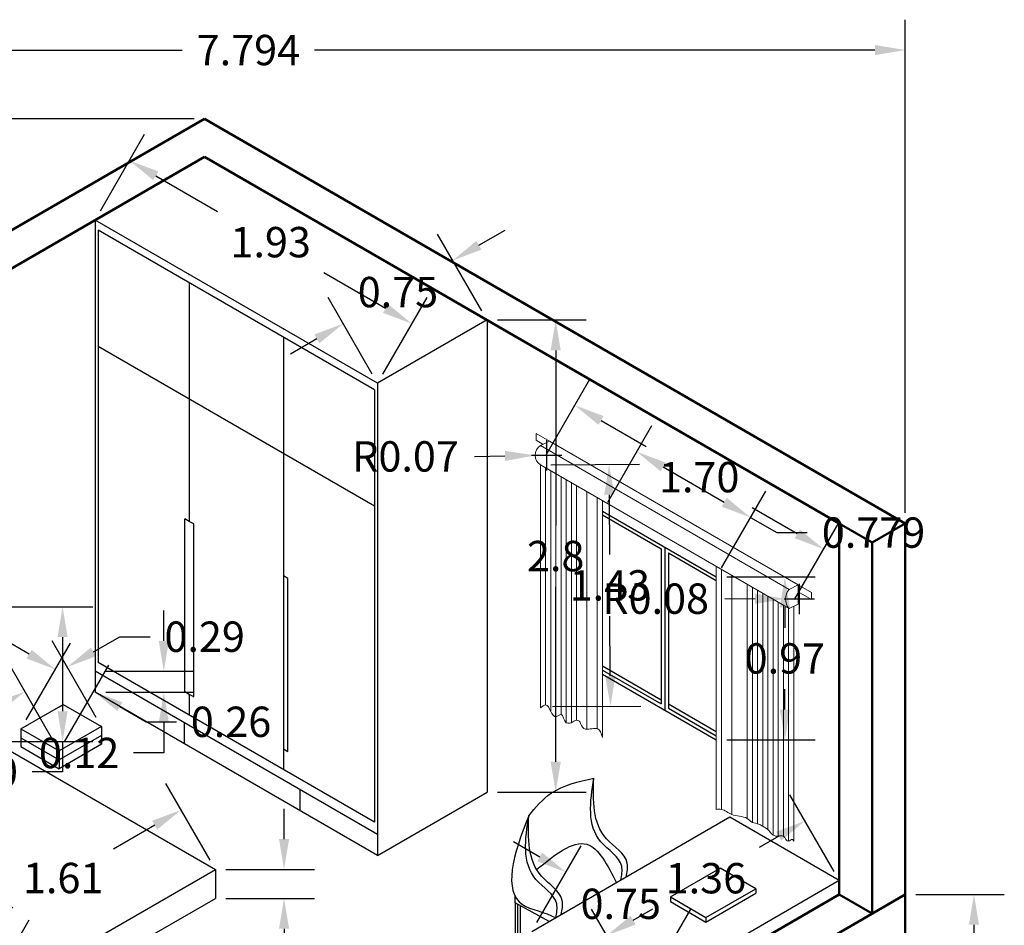
# Model space of a CAD drawing. Units: metres. Extents: x 4633 to 4644.7, y 5356.8 to 5365.2.
# Tile 3 of 3: x 4638.8 to 4644.7, y 5359.9 to 5365.2. Entities that reach past the tile are written whole.
import ezdxf

# ---------------------------------------------------------------- set-up
doc = ezdxf.new("R2010")
doc.units = ezdxf.units.M
for name, color, linetype, lineweight in [('A-ANNO-DIMS', 2, 'Continuous', 18), ('A-FURN', 8, 'Continuous', 25), ('A-FURN-CURT', 8, 'Continuous', 18), ('A-GLAZ', 4, 'Continuous', 25), ('A-WALL', 7, 'Continuous', 50)]:
    doc.layers.add(name, color=color, linetype=linetype, lineweight=lineweight)
doc.styles.get("Standard").update_dxf_attribs({"font": 'arial.ttf'})
doc.dimstyles.get("Standard").update_dxf_attribs({"dimtxt": 0.18, "dimasz": 0.18, "dimexe": 0.18, "dimexo": 0.0625, "dimgap": 0.09, "dimtad": 0, "dimtih": 1, "dimtoh": 1, "dimdec": 4, "dimzin": 0, "dimdsep": 46, "dimtxsty": 'Standard', "dimcen": 0.09, "dimadec": 0, "dimazin": 0, "dimtfac": 1, "dimtdec": 4, "dimtofl": 0, "dimtmove": 0, "dimatfit": 3, "dimfxl": 1, "dimtolj": 1, "dimtzin": 0, "dimarcsym": 0})

# ---------------------------------------------------------------- blocks, each defined once
blk = doc.blocks.new('*D2')
at = {"layer": 'A-ANNO-DIMS', "color": 0, "lineweight": -2, "transparency": 16777216}
for p, q in [((4636.2802, 5362.6038), (4636.2802, 5365.2288)), ((4644.0744, 5362.3038), (4644.0744, 5365.2288)), ((4636.4602, 5365.0488), (4639.7847, 5365.0488)), ((4643.8944, 5365.0488), (4640.5699, 5365.0488))]:
    blk.add_line(p, q, dxfattribs=at)
at = {"layer": 'A-ANNO-DIMS', "color": 0, "transparency": 16777216}
for points in [[(4636.4602, 5365.0788), (4636.4602, 5365.0188), (4636.2802, 5365.0488)], [(4643.8944, 5365.0788), (4643.8944, 5365.0188), (4644.0744, 5365.0488)]]:
    blk.add_solid(points, dxfattribs=at)
at = {"layer": 'Defpoints', "color": 0, "transparency": 16777216}
for p in [(4644.0744, 5365.0488), (4636.2802, 5362.5413), (4644.0744, 5362.2413)]:
    blk.add_point(p, dxfattribs=at)
at = {"layer": 'A-ANNO-DIMS', "color": 0, "transparency": 16777216, "insert": (4640.1773, 5365.0488), "char_height": 0.18, "attachment_point": 5}
blk.add_mtext('\\A1;7.794', dxfattribs=at)
blk = doc.blocks.new('*D3')
at = {"layer": 'A-ANNO-DIMS', "color": 0, "lineweight": -2, "transparency": 16777216}
for p, q in [((4639.855, 5364.6413), (4635.6927, 5364.6413)), ((4635.8727, 5364.4613), (4635.8727, 5360.9232)), ((4635.8727, 5357.0213), (4635.8727, 5360.5594)), ((4639.855, 5356.8413), (4635.6927, 5356.8413))]:
    blk.add_line(p, q, dxfattribs=at)
at = {"layer": 'A-ANNO-DIMS', "color": 0, "transparency": 16777216}
for points in [[(4635.8427, 5364.4613), (4635.9027, 5364.4613), (4635.8727, 5364.6413)], [(4635.8427, 5357.0213), (4635.9027, 5357.0213), (4635.8727, 5356.8413)]]:
    blk.add_solid(points, dxfattribs=at)
at = {"layer": 'Defpoints', "color": 0, "transparency": 16777216}
for p in [(4639.9175, 5364.6413), (4635.8727, 5356.8413), (4639.9175, 5356.8413)]:
    blk.add_point(p, dxfattribs=at)
at = {"layer": 'A-ANNO-DIMS', "color": 0, "transparency": 16777216, "insert": (4635.8727, 5360.7413), "char_height": 0.18, "attachment_point": 5}
blk.add_mtext('\\A1;7.8', dxfattribs=at)
blk = doc.blocks.new('*D6')
at = {"layer": 'A-ANNO-DIMS', "color": 0, "lineweight": -2, "transparency": 16777216}
for p, q in [((4644.1369, 5360.0413), (4644.6619, 5360.0413)), ((4644.4819, 5359.8613), (4644.4819, 5359.4213)), ((4644.1369, 5359.2413), (4644.6619, 5359.2413)), ((4644.4819, 5359.2413), (4644.4819, 5359.0613)), ((4644.4819, 5359.0613), (4644.3019, 5359.0613))]:
    blk.add_line(p, q, dxfattribs=at)
at = {"layer": 'A-ANNO-DIMS', "color": 0, "transparency": 16777216}
for points in [[(4644.4519, 5359.8613), (4644.5119, 5359.8613), (4644.4819, 5360.0413)], [(4644.4519, 5359.4213), (4644.5119, 5359.4213), (4644.4819, 5359.2413)]]:
    blk.add_solid(points, dxfattribs=at)
at = {"layer": 'Defpoints', "color": 0, "transparency": 16777216}
for p in [(4644.0744, 5360.0413), (4644.0744, 5359.2413), (4644.4819, 5359.2413)]:
    blk.add_point(p, dxfattribs=at)
at = {"layer": 'A-ANNO-DIMS', "color": 0, "transparency": 16777216, "insert": (4644.0479, 5359.0613), "char_height": 0.18, "attachment_point": 5}
blk.add_mtext('\\A1;0.8', dxfattribs=at)
blk = doc.blocks.new('*D9')
at = {"layer": 'A-ANNO-DIMS', "color": 0, "lineweight": -2, "transparency": 16777216}
for p, q in [((4642.309, 5362.3679), (4642.5715, 5362.8225)), ((4642.6374, 5362.5767), (4643.0003, 5362.3671)), ((4642.9837, 5361.9783), (4643.2462, 5362.433)), ((4643.1562, 5362.2771), (4643.3121, 5362.1871)), ((4643.3121, 5362.1871), (4643.4921, 5362.1871))]:
    blk.add_line(p, q, dxfattribs=at)
at = {"layer": 'A-ANNO-DIMS', "color": 0, "transparency": 16777216}
for points in [[(4642.6524, 5362.6026), (4642.6224, 5362.5507), (4642.4815, 5362.6667)], [(4643.0153, 5362.3931), (4642.9853, 5362.3411), (4643.1562, 5362.2771)]]:
    blk.add_solid(points, dxfattribs=at)
at = {"layer": 'Defpoints', "color": 0, "transparency": 16777216}
for p in [(4642.2778, 5362.3137), (4643.1562, 5362.2771), (4642.9525, 5361.9242)]:
    blk.add_point(p, dxfattribs=at)
at = {"layer": 'A-ANNO-DIMS', "color": 0, "transparency": 16777216, "insert": (4643.886, 5362.1871), "char_height": 0.18, "attachment_point": 5}
blk.add_mtext('\\A1;0.779', dxfattribs=at)
blk = doc.blocks.new('*D10')
at = {"layer": 'A-ANNO-DIMS', "color": 0, "lineweight": -2, "transparency": 16777216}
for p, q in [((4643.015, 5361.9242), (4643.54, 5361.9242)), ((4643.36, 5361.7442), (4643.36, 5361.6227)), ((4643.36, 5361.1374), (4643.36, 5361.2589)), ((4643.015, 5360.9574), (4643.54, 5360.9574))]:
    blk.add_line(p, q, dxfattribs=at)
at = {"layer": 'A-ANNO-DIMS', "color": 0, "transparency": 16777216}
for points in [[(4643.33, 5361.7442), (4643.39, 5361.7442), (4643.36, 5361.9242)], [(4643.33, 5361.1374), (4643.39, 5361.1374), (4643.36, 5360.9574)]]:
    blk.add_solid(points, dxfattribs=at)
at = {"layer": 'Defpoints', "color": 0, "transparency": 16777216}
for p in [(4642.9525, 5361.9242), (4642.9525, 5360.9574), (4643.36, 5360.9574)]:
    blk.add_point(p, dxfattribs=at)
at = {"layer": 'A-ANNO-DIMS', "color": 0, "transparency": 16777216, "insert": (4643.36, 5361.4408), "char_height": 0.18, "attachment_point": 5}
blk.add_mtext('\\A1;0.97', dxfattribs=at)
blk = doc.blocks.new('*D11')
at = {"layer": 'A-ANNO-DIMS', "color": 0, "lineweight": -2, "transparency": 16777216}
for p, q in [((4641.9722, 5362.5896), (4642.4972, 5362.5926)), ((4642.3183, 5362.4116), (4642.3203, 5362.0563)), ((4642.3243, 5361.337), (4642.3223, 5361.6923)), ((4641.9804, 5361.1551), (4642.5054, 5361.158))]:
    blk.add_line(p, q, dxfattribs=at)
at = {"layer": 'A-ANNO-DIMS', "color": 0, "transparency": 16777216}
for points in [[(4642.3483, 5362.4117), (4642.2883, 5362.4114), (4642.3172, 5362.5916)], [(4642.3543, 5361.3372), (4642.2943, 5361.3368), (4642.3254, 5361.157)]]:
    blk.add_solid(points, dxfattribs=at)
at = {"layer": 'Defpoints', "color": 0, "transparency": 16777216}
for p in [(4641.9097, 5362.5893), (4642.3254, 5361.157), (4641.9179, 5361.1547)]:
    blk.add_point(p, dxfattribs=at)
at = {"layer": 'A-ANNO-DIMS', "color": 0, "transparency": 16777216, "insert": (4642.3213, 5361.8743), "char_height": 0.18, "attachment_point": 5}
blk.add_mtext('\\A1;1.43', dxfattribs=at)
blk = doc.blocks.new('*D12')
at = {"layer": 'A-ANNO-DIMS', "color": 0, "lineweight": -2, "transparency": 16777216}
for p, q in [((4641.941, 5362.6434), (4642.2035, 5363.098)), ((4642.2694, 5362.8522), (4642.5366, 5362.6979)), ((4643.4339, 5362.1798), (4643.1666, 5362.3341)), ((4643.4173, 5361.791), (4643.6798, 5362.2457))]:
    blk.add_line(p, q, dxfattribs=at)
at = {"layer": 'A-ANNO-DIMS', "color": 0, "transparency": 16777216}
for points in [[(4642.2844, 5362.8781), (4642.2544, 5362.8262), (4642.1135, 5362.9422)], [(4643.4489, 5362.2058), (4643.4189, 5362.1538), (4643.5898, 5362.0898)]]:
    blk.add_solid(points, dxfattribs=at)
at = {"layer": 'Defpoints', "color": 0, "transparency": 16777216}
for p in [(4641.9097, 5362.5893), (4643.5898, 5362.0898), (4643.386, 5361.7369)]:
    blk.add_point(p, dxfattribs=at)
at = {"layer": 'A-ANNO-DIMS', "color": 0, "transparency": 16777216, "insert": (4642.8516, 5362.516), "char_height": 0.18, "attachment_point": 5}
blk.add_mtext('\\A1;1.70', dxfattribs=at)
blk = doc.blocks.new('*D13')
at = {"layer": 'A-ANNO-DIMS', "color": 0, "lineweight": -2, "transparency": 16777216}
for p, q in [((4639.2992, 5364.0944), (4639.5617, 5364.5491)), ((4639.6276, 5364.3032), (4639.9942, 5364.0915)), ((4640.9911, 5363.516), (4640.6245, 5363.7276)), ((4640.9745, 5363.1272), (4641.237, 5363.5818))]:
    blk.add_line(p, q, dxfattribs=at)
at = {"layer": 'A-ANNO-DIMS', "color": 0, "transparency": 16777216}
for points in [[(4639.6426, 5364.3292), (4639.6126, 5364.2772), (4639.4717, 5364.3932)], [(4641.0061, 5363.5419), (4640.9761, 5363.49), (4641.147, 5363.426)]]:
    blk.add_solid(points, dxfattribs=at)
at = {"layer": 'Defpoints', "color": 0, "transparency": 16777216}
for p in [(4639.268, 5364.0403), (4641.147, 5363.426), (4640.9433, 5363.073)]:
    blk.add_point(p, dxfattribs=at)
at = {"layer": 'A-ANNO-DIMS', "color": 0, "transparency": 16777216, "insert": (4640.3094, 5363.9096), "char_height": 0.18, "attachment_point": 5}
blk.add_mtext('\\A1;1.93', dxfattribs=at)
blk = doc.blocks.new('*D14')
at = {"layer": 'A-ANNO-DIMS', "color": 0, "lineweight": -2, "transparency": 16777216}
for p, q in [((4641.5449, 5363.891), (4641.7008, 5363.981)), ((4641.5615, 5363.5022), (4641.299, 5363.9568)), ((4640.912, 5363.1272), (4640.6495, 5363.5818)), ((4640.5836, 5363.336), (4640.4277, 5363.246))]:
    blk.add_line(p, q, dxfattribs=at)
at = {"layer": 'A-ANNO-DIMS', "color": 0, "transparency": 16777216}
for points in [[(4641.5299, 5363.9169), (4641.5599, 5363.865), (4641.389, 5363.801)], [(4640.5686, 5363.3619), (4640.5986, 5363.31), (4640.7395, 5363.426)]]:
    blk.add_solid(points, dxfattribs=at)
at = {"layer": 'Defpoints', "color": 0, "transparency": 16777216}
for p in [(4641.389, 5363.801), (4641.5928, 5363.448), (4640.9433, 5363.073)]:
    blk.add_point(p, dxfattribs=at)
at = {"layer": 'A-ANNO-DIMS', "color": 0, "transparency": 16777216, "insert": (4641.0643, 5363.6135), "char_height": 0.18, "attachment_point": 5}
blk.add_mtext('\\A1;0.75', dxfattribs=at)
blk = doc.blocks.new('*D15')
at = {"layer": 'A-ANNO-DIMS', "color": 0, "lineweight": -2, "transparency": 16777216}
for p, q in [((4641.6553, 5363.448), (4642.1803, 5363.448)), ((4642.0003, 5363.268), (4642.0003, 5362.23)), ((4642.0003, 5360.828), (4642.0003, 5361.8661)), ((4641.6553, 5360.648), (4642.1803, 5360.648))]:
    blk.add_line(p, q, dxfattribs=at)
at = {"layer": 'A-ANNO-DIMS', "color": 0, "transparency": 16777216}
for points in [[(4641.9703, 5363.268), (4642.0303, 5363.268), (4642.0003, 5363.448)], [(4641.9703, 5360.828), (4642.0303, 5360.828), (4642.0003, 5360.648)]]:
    blk.add_solid(points, dxfattribs=at)
at = {"layer": 'Defpoints', "color": 0, "transparency": 16777216}
for p in [(4641.5928, 5363.448), (4641.5928, 5360.648), (4642.0003, 5360.648)]:
    blk.add_point(p, dxfattribs=at)
at = {"layer": 'A-ANNO-DIMS', "color": 0, "transparency": 16777216, "insert": (4642.0003, 5362.048), "char_height": 0.18, "attachment_point": 5}
blk.add_mtext('\\A1;2.8', dxfattribs=at)
blk = doc.blocks.new('*D16')
at = {"layer": 'A-ANNO-DIMS', "color": 0, "lineweight": -2, "transparency": 16777216}
for p, q in [((4639.6755, 5361.545), (4639.6755, 5361.725)), ((4639.3305, 5361.365), (4639.8555, 5361.365)), ((4639.3305, 5361.2403), (4639.8555, 5361.2403)), ((4639.6755, 5361.0603), (4639.6755, 5360.8803)), ((4639.6755, 5360.8803), (4639.4955, 5360.8803))]:
    blk.add_line(p, q, dxfattribs=at)
at = {"layer": 'A-ANNO-DIMS', "color": 0, "transparency": 16777216}
for points in [[(4639.6455, 5361.545), (4639.7055, 5361.545), (4639.6755, 5361.365)], [(4639.6455, 5361.0603), (4639.7055, 5361.0603), (4639.6755, 5361.2403)]]:
    blk.add_solid(points, dxfattribs=at)
at = {"layer": 'Defpoints', "color": 0, "transparency": 16777216}
for p in [(4639.268, 5361.365), (4639.268, 5361.2403), (4639.6755, 5361.2403)]:
    blk.add_point(p, dxfattribs=at)
at = {"layer": 'A-ANNO-DIMS', "color": 0, "transparency": 16777216, "insert": (4639.1726, 5360.8803), "char_height": 0.18, "attachment_point": 5}
blk.add_mtext('\\A1;0.12', dxfattribs=at)
blk = doc.blocks.new('*D17')
at = {"layer": 'A-ANNO-DIMS', "color": 0, "lineweight": -2, "transparency": 16777216}
for p, q in [((4637.213, 5360.2454), (4637.4755, 5360.7001)), ((4637.5414, 5360.4542), (4637.771, 5360.3216)), ((4638.6308, 5359.8252), (4638.4012, 5359.9578)), ((4638.6142, 5359.4364), (4638.8767, 5359.8911))]:
    blk.add_line(p, q, dxfattribs=at)
at = {"layer": 'A-ANNO-DIMS', "color": 0, "transparency": 16777216}
for points in [[(4637.5564, 5360.4802), (4637.5264, 5360.4282), (4637.3855, 5360.5442)], [(4638.6458, 5359.8512), (4638.6158, 5359.7992), (4638.7867, 5359.7352)]]:
    blk.add_solid(points, dxfattribs=at)
at = {"layer": 'Defpoints', "color": 0, "transparency": 16777216}
for p in [(4637.1817, 5360.1913), (4638.7867, 5359.7352), (4638.583, 5359.3823)]:
    blk.add_point(p, dxfattribs=at)
at = {"layer": 'A-ANNO-DIMS', "color": 0, "transparency": 16777216, "insert": (4638.0861, 5360.1397), "char_height": 0.18, "attachment_point": 5}
blk.add_mtext('\\A1;1.618', dxfattribs=at)
blk = doc.blocks.new('*D18')
at = {"layer": 'A-ANNO-DIMS', "color": 0, "lineweight": -2, "transparency": 16777216}
for p, q in [((4639.9499, 5360.2437), (4639.6874, 5360.6983)), ((4639.6215, 5360.4524), (4639.3762, 5360.3108)), ((4638.5351, 5359.8252), (4638.7804, 5359.9668)), ((4638.5517, 5359.4364), (4638.2892, 5359.8911))]:
    blk.add_line(p, q, dxfattribs=at)
at = {"layer": 'A-ANNO-DIMS', "color": 0, "transparency": 16777216}
for points in [[(4639.6065, 5360.4784), (4639.6365, 5360.4265), (4639.7774, 5360.5424)], [(4638.5201, 5359.8512), (4638.5501, 5359.7992), (4638.3792, 5359.7352)]]:
    blk.add_solid(points, dxfattribs=at)
at = {"layer": 'Defpoints', "color": 0, "transparency": 16777216}
for p in [(4639.7774, 5360.5424), (4639.9812, 5360.1895), (4638.583, 5359.3823)]:
    blk.add_point(p, dxfattribs=at)
at = {"layer": 'A-ANNO-DIMS', "color": 0, "transparency": 16777216, "insert": (4639.0783, 5360.1388), "char_height": 0.18, "attachment_point": 5}
blk.add_mtext('\\A1;1.61', dxfattribs=at)
blk = doc.blocks.new('*D19')
at = {"layer": 'A-ANNO-DIMS', "color": 0, "lineweight": -2, "transparency": 16777216}
for p, q in [((4640.3887, 5360.3695), (4640.3887, 5360.5495)), ((4640.0437, 5360.1895), (4640.5687, 5360.1895)), ((4640.0437, 5360.0182), (4640.5687, 5360.0182)), ((4640.3887, 5359.8382), (4640.3887, 5359.6582)), ((4640.3887, 5359.6582), (4640.2087, 5359.6582))]:
    blk.add_line(p, q, dxfattribs=at)
at = {"layer": 'A-ANNO-DIMS', "color": 0, "transparency": 16777216}
for points in [[(4640.3587, 5360.3695), (4640.4187, 5360.3695), (4640.3887, 5360.1895)], [(4640.3587, 5359.8382), (4640.4187, 5359.8382), (4640.3887, 5360.0182)]]:
    blk.add_solid(points, dxfattribs=at)
at = {"layer": 'Defpoints', "color": 0, "transparency": 16777216}
for p in [(4639.9812, 5360.1895), (4639.9812, 5360.0182), (4640.3887, 5360.0182)]:
    blk.add_point(p, dxfattribs=at)
at = {"layer": 'A-ANNO-DIMS', "color": 0, "transparency": 16777216, "insert": (4639.8849, 5359.6582), "char_height": 0.18, "attachment_point": 5}
blk.add_mtext('\\A1;0.17', dxfattribs=at)
blk = doc.blocks.new('*D20')
at = {"layer": 'A-ANNO-DIMS', "color": 0, "lineweight": -2, "transparency": 16777216}
for p, q in [((4638.7298, 5361.7474), (4639.2548, 5361.7474)), ((4639.0748, 5361.5674), (4639.0748, 5361.1281)), ((4638.7298, 5360.9481), (4639.2548, 5360.9481)), ((4639.0748, 5360.9481), (4639.0748, 5360.7681)), ((4639.0748, 5360.7681), (4638.8948, 5360.7681))]:
    blk.add_line(p, q, dxfattribs=at)
at = {"layer": 'A-ANNO-DIMS', "color": 0, "transparency": 16777216}
for points in [[(4639.0448, 5361.5674), (4639.1048, 5361.5674), (4639.0748, 5361.7474)], [(4639.0448, 5361.1281), (4639.1048, 5361.1281), (4639.0748, 5360.9481)]]:
    blk.add_solid(points, dxfattribs=at)
at = {"layer": 'Defpoints', "color": 0, "transparency": 16777216}
for p in [(4638.6673, 5361.7474), (4638.6673, 5360.9481), (4639.0748, 5360.9481)]:
    blk.add_point(p, dxfattribs=at)
at = {"layer": 'A-ANNO-DIMS', "color": 0, "transparency": 16777216, "insert": (4638.5714, 5360.7681), "char_height": 0.18, "attachment_point": 5}
blk.add_mtext('\\A1;0.80', dxfattribs=at)
blk = doc.blocks.new('*D22')
at = {"layer": 'A-ANNO-DIMS', "color": 0, "lineweight": -2, "transparency": 16777216}
for p, q in [((4638.8758, 5361.4662), (4638.7199, 5361.5562)), ((4638.8591, 5361.0775), (4639.1216, 5361.5321)), ((4639.0863, 5360.9463), (4639.3488, 5361.401)), ((4639.4147, 5361.1551), (4639.5706, 5361.0651)), ((4639.5706, 5361.0651), (4639.7506, 5361.0651))]:
    blk.add_line(p, q, dxfattribs=at)
at = {"layer": 'A-ANNO-DIMS', "color": 0, "transparency": 16777216}
for points in [[(4638.8908, 5361.4922), (4638.8608, 5361.4403), (4639.0316, 5361.3762)], [(4639.4297, 5361.1811), (4639.3997, 5361.1291), (4639.2588, 5361.2451)]]:
    blk.add_solid(points, dxfattribs=at)
at = {"layer": 'Defpoints', "color": 0, "transparency": 16777216}
for p in [(4639.2588, 5361.2451), (4638.8279, 5361.0233), (4639.0551, 5360.8922)]:
    blk.add_point(p, dxfattribs=at)
at = {"layer": 'A-ANNO-DIMS', "color": 0, "transparency": 16777216, "insert": (4640.0743, 5361.0651), "char_height": 0.18, "attachment_point": 5}
blk.add_mtext('\\A1;0.26', dxfattribs=at)
blk = doc.blocks.new('*D23')
at = {"layer": 'A-ANNO-DIMS', "color": 0, "lineweight": -2, "transparency": 16777216}
for p, q in [((4639.258, 5361.4799), (4639.4139, 5361.5699)), ((4639.4139, 5361.5699), (4639.5939, 5361.5699)), ((4639.2746, 5361.0911), (4639.0121, 5361.5457)), ((4639.0238, 5360.9463), (4638.7613, 5361.401)), ((4638.6954, 5361.1551), (4638.5395, 5361.0651))]:
    blk.add_line(p, q, dxfattribs=at)
at = {"layer": 'A-ANNO-DIMS', "color": 0, "transparency": 16777216}
for points in [[(4639.243, 5361.5058), (4639.273, 5361.4539), (4639.1021, 5361.3899)], [(4638.6804, 5361.1811), (4638.7104, 5361.1291), (4638.8513, 5361.2451)]]:
    blk.add_solid(points, dxfattribs=at)
at = {"layer": 'Defpoints', "color": 0, "transparency": 16777216}
for p in [(4639.1021, 5361.3899), (4639.3058, 5361.037), (4639.0551, 5360.8922)]:
    blk.add_point(p, dxfattribs=at)
at = {"layer": 'A-ANNO-DIMS', "color": 0, "transparency": 16777216, "insert": (4639.9178, 5361.5699), "char_height": 0.18, "attachment_point": 5}
blk.add_mtext('\\A1;0.29', dxfattribs=at)
blk = doc.blocks.new('*D25')
at = {"layer": 'A-ANNO-DIMS', "color": 0, "lineweight": -2, "transparency": 16777216}
for p, q in [((4641.9058, 5360.2632), (4641.7499, 5360.3532)), ((4641.8892, 5359.8745), (4642.1517, 5360.3291)), ((4642.5387, 5359.4995), (4642.8012, 5359.9541)), ((4642.8671, 5359.7082), (4643.023, 5359.6182))]:
    blk.add_line(p, q, dxfattribs=at)
at = {"layer": 'A-ANNO-DIMS', "color": 0, "transparency": 16777216}
for points in [[(4641.9208, 5360.2892), (4641.8908, 5360.2373), (4642.0617, 5360.1732)], [(4642.8821, 5359.7342), (4642.8521, 5359.6823), (4642.7112, 5359.7982)]]:
    blk.add_solid(points, dxfattribs=at)
at = {"layer": 'Defpoints', "color": 0, "transparency": 16777216}
for p in [(4641.8579, 5359.8203), (4642.7112, 5359.7982), (4642.5075, 5359.4453)]:
    blk.add_point(p, dxfattribs=at)
at = {"layer": 'A-ANNO-DIMS', "color": 0, "transparency": 16777216, "insert": (4642.3865, 5359.9857), "char_height": 0.18, "attachment_point": 5}
blk.add_mtext('\\A1;0.75', dxfattribs=at)
blk = doc.blocks.new('*D26')
at = {"layer": 'A-ANNO-DIMS', "color": 0, "lineweight": -2, "transparency": 16777216}
for p, q in [((4643.6517, 5360.1781), (4643.3892, 5360.6328)), ((4643.3233, 5360.3869), (4643.2066, 5360.3195)), ((4642.4762, 5359.4995), (4642.2137, 5359.9541)), ((4642.4596, 5359.8882), (4642.5763, 5359.9556))]:
    blk.add_line(p, q, dxfattribs=at)
at = {"layer": 'A-ANNO-DIMS', "color": 0, "transparency": 16777216}
for points in [[(4643.3083, 5360.4129), (4643.3383, 5360.3609), (4643.4792, 5360.4769)], [(4642.4446, 5359.9142), (4642.4746, 5359.8623), (4642.3037, 5359.7982)]]:
    blk.add_solid(points, dxfattribs=at)
at = {"layer": 'Defpoints', "color": 0, "transparency": 16777216}
for p in [(4643.4792, 5360.4769), (4643.683, 5360.124), (4642.5075, 5359.4453)]:
    blk.add_point(p, dxfattribs=at)
at = {"layer": 'A-ANNO-DIMS', "color": 0, "transparency": 16777216, "insert": (4642.8915, 5360.1376), "char_height": 0.18, "attachment_point": 5}
blk.add_mtext('\\A1;1.36', dxfattribs=at)
blk = doc.blocks.new('*D30')
at = {"layer": 'A-ANNO-DIMS', "color": 0, "lineweight": -2, "transparency": 16777216}
for p, q in [((4633.8236, 5361.0144), (4634.0036, 5361.0144)), ((4634.0036, 5361.0144), (4636.779, 5359.9989)), ((4641.8554, 5358.0514), (4641.8554, 5358.2314)), ((4641.7654, 5358.1414), (4641.9454, 5358.1414))]:
    blk.add_line(p, q, dxfattribs=at)
at = {"layer": 'A-ANNO-DIMS', "color": 0, "transparency": 16777216}
blk.add_solid([(4636.7893, 5360.027), (4636.7686, 5359.9707), (4636.948, 5359.937)], dxfattribs=at)
at = {"layer": 'Defpoints', "color": 0, "transparency": 16777216}
for p in [(4636.948, 5359.937), (4641.8554, 5358.1414)]:
    blk.add_point(p, dxfattribs=at)
at = {"layer": 'A-ANNO-DIMS', "color": 0, "transparency": 16777216, "insert": (4633.3438, 5361.0144), "char_height": 0.18, "attachment_point": 5}
blk.add_mtext('\\A1;R5.226', dxfattribs=at)
blk = doc.blocks.new('*D32')
at = {"layer": 'A-ANNO-DIMS', "color": 0, "lineweight": -2, "transparency": 16777216}
for p, q in [((4643.4464, 5361.7037), (4643.4464, 5361.8837)), ((4643.0035, 5361.7954), (4643.1835, 5361.7947)), ((4643.3564, 5361.7937), (4643.5364, 5361.7937))]:
    blk.add_line(p, q, dxfattribs=at)
at = {"layer": 'A-ANNO-DIMS', "color": 0, "transparency": 16777216}
blk.add_solid([(4643.1837, 5361.8247), (4643.1834, 5361.7647), (4643.3635, 5361.794)], dxfattribs=at)
at = {"layer": 'Defpoints', "color": 0, "transparency": 16777216}
for p in [(4643.3635, 5361.794), (4643.4464, 5361.7937)]:
    blk.add_point(p, dxfattribs=at)
at = {"layer": 'A-ANNO-DIMS', "color": 0, "transparency": 16777216, "insert": (4642.5935, 5361.7954), "char_height": 0.18, "attachment_point": 5}
blk.add_mtext('\\A1;R0.08', dxfattribs=at)
blk = doc.blocks.new('*D33')
at = {"layer": 'A-ANNO-DIMS', "color": 0, "lineweight": -2, "transparency": 16777216}
for p, q in [((4641.947, 5362.556), (4641.947, 5362.736)), ((4641.5191, 5362.6391), (4641.6991, 5362.642)), ((4641.857, 5362.646), (4642.037, 5362.646))]:
    blk.add_line(p, q, dxfattribs=at)
at = {"layer": 'A-ANNO-DIMS', "color": 0, "transparency": 16777216}
blk.add_solid([(4641.6986, 5362.672), (4641.6996, 5362.612), (4641.8791, 5362.6449)], dxfattribs=at)
at = {"layer": 'Defpoints', "color": 0, "transparency": 16777216}
for p in [(4641.8791, 5362.6449), (4641.947, 5362.646)]:
    blk.add_point(p, dxfattribs=at)
at = {"layer": 'A-ANNO-DIMS', "color": 0, "transparency": 16777216, "insert": (4641.1092, 5362.6391), "char_height": 0.18, "attachment_point": 5}
blk.add_mtext('\\A1;R0.07', dxfattribs=at)

msp = doc.modelspace()

# ---------------------------------------------------------------- linework, layer by layer
at = {"layer": 'A-FURN'}
for p, q in [((4640.9433, 5363.073), (4639.268, 5364.0403)), ((4639.268, 5364.0403), (4639.268, 5361.2403)), ((4639.2853, 5363.9803), (4639.2853, 5361.4165)), ((4640.9259, 5363.033), (4639.2853, 5363.9803)), ((4639.8264, 5363.6679), (4639.8264, 5362.2537)), ((4641.5928, 5363.448), (4640.9433, 5363.073)), ((4641.5928, 5363.448), (4641.5928, 5360.648)), ((4640.3848, 5363.3455), (4640.3848, 5360.7817)), ((4640.9259, 5362.3435), (4639.2853, 5363.2907)), ((4640.9259, 5363.033), (4640.9259, 5360.4693)), ((4640.9433, 5363.073), (4640.9433, 5360.273)), ((4639.7998, 5361.244), (4639.7998, 5362.2691)), ((4639.8264, 5362.2537), (4639.7998, 5362.2691)), ((4639.853, 5362.2383), (4639.8264, 5362.2537)), ((4639.853, 5361.2133), (4639.853, 5362.2383)), ((4640.4115, 5361.9145), (4640.3848, 5361.9299)), ((4640.4115, 5360.8895), (4640.4115, 5361.9145)), ((4640.9259, 5360.4693), (4639.2853, 5361.4165)), ((4640.9433, 5360.3977), (4639.268, 5361.365)), ((4640.9433, 5360.273), (4639.268, 5361.2403)), ((4639.7998, 5361.244), (4639.8264, 5361.2286)), ((4639.8264, 5361.2286), (4639.853, 5361.2133)), ((4639.8264, 5361.2286), (4639.8264, 5361.1041)), ((4638.8279, 5361.0233), (4639.0787, 5361.1681)), ((4639.055, 5361.1544), (4639.0787, 5361.1681)), ((4639.0787, 5361.1681), (4639.3058, 5361.037)), ((4639.7952, 5361.0606), (4639.7952, 5360.9359)), ((4638.8279, 5361.0233), (4639.0551, 5360.8922)), ((4638.8279, 5361.0233), (4638.8279, 5360.9707)), ((4639.3058, 5361.037), (4639.0551, 5360.8922)), ((4639.3058, 5360.9843), (4639.0551, 5360.8395)), ((4639.3058, 5360.9843), (4639.0551, 5360.8395)), ((4639.3058, 5361.037), (4639.3058, 5360.9843)), ((4639.3058, 5360.9843), (4639.3058, 5360.9316)), ((4638.6673, 5360.9481), (4639.9812, 5360.1895)), ((4638.8279, 5360.9707), (4639.0551, 5360.8395)), ((4638.8279, 5360.9707), (4639.0551, 5360.8395)), ((4638.8279, 5360.9707), (4638.8279, 5360.918)), ((4639.3058, 5360.9316), (4639.0551, 5360.7868)), ((4638.8279, 5360.918), (4639.0551, 5360.7868)), ((4639.0551, 5360.8922), (4639.0551, 5360.8395)), ((4640.3848, 5360.9049), (4640.4115, 5360.8895)), ((4639.0551, 5360.8395), (4639.0551, 5360.7868)), ((4640.4816, 5360.6643), (4640.4816, 5360.5396)), ((4640.9433, 5360.273), (4641.5928, 5360.648)), ((4643.0334, 5360.499), (4641.8579, 5359.8203)), ((4643.683, 5360.124), (4643.0334, 5360.499)), ((4638.583, 5359.3823), (4639.9812, 5360.1895)), ((4639.9812, 5360.1895), (4639.9812, 5360.0182)), ((4642.6809, 5360.0264), (4642.977, 5360.1974)), ((4643.1881, 5360.0755), (4642.977, 5360.1974)), ((4643.683, 5360.124), (4642.5075, 5359.4453)), ((4642.892, 5359.9046), (4643.1881, 5360.0755)), ((4642.892, 5359.8772), (4643.1881, 5360.0481)), ((4643.1881, 5360.0755), (4643.1881, 5360.0481)), ((4638.583, 5359.2109), (4639.9812, 5360.0182)), ((4641.7594, 5359.9907), (4641.7594, 5360.0309)), ((4641.9624, 5359.8807), (4641.7594, 5359.9907)), ((4641.7594, 5359.9907), (4641.7594, 5359.388)), ((4642.6809, 5360.0264), (4642.892, 5359.9046)), ((4642.6809, 5360.0264), (4642.6809, 5359.999)), ((4642.6809, 5359.999), (4642.892, 5359.8772)), ((4641.7751, 5359.3789), (4641.7751, 5359.9822)), ((4641.7922, 5359.3888), (4641.7922, 5359.9729)), ((4642.892, 5359.9046), (4642.892, 5359.8772))]:
    msp.add_line(p, q, dxfattribs=at)
for points, knots in [([(4641.8405, 5360.5081), (4641.8815, 5360.5573), (4641.9812, 5360.677), (4642.1353, 5360.7108), (4642.226, 5360.7306)], [0, 0, 0, 0, 0.1876846, 0.4562802, 0.4562802, 0.4562802, 0.4562802]), ([(4642.3862, 5360.1253), (4642.3918, 5360.1543), (4642.4101, 5360.2492), (4642.1738, 5360.3809), (4642.2051, 5360.5907), (4642.226, 5360.7306)], [0, 0, 0, 0, 0.0833387, 0.2733856, 0.6532652, 0.6532652, 0.6532652, 0.6532652]), ([(4642.419, 5360.1443), (4642.4245, 5360.1732), (4642.4426, 5360.2681), (4642.215, 5360.3974), (4642.2216, 5360.5983), (4642.226, 5360.7306)], [0, 0, 0, 0, 0.0833387, 0.2733856, 0.6398086, 0.6398086, 0.6398086, 0.6398086]), ([(4641.8405, 5360.5081), (4641.7468, 5360.2759), (4641.6606, 5359.9691), (4641.9342, 5359.9397), (4642.0007, 5359.9028)], [0, 0, 0, 0, 0.5391492, 0.7667446, 0.7667446, 0.7667446, 0.7667446]), ([(4642.0007, 5359.9028), (4642.0063, 5359.9317), (4642.0245, 5360.0267), (4641.7883, 5360.1583), (4641.8196, 5360.3682), (4641.8405, 5360.5081)], [0, 0, 0, 0, 0.0833387, 0.2733856, 0.6532652, 0.6532652, 0.6532652, 0.6532652]), ([(4642.0335, 5359.9217), (4642.039, 5359.9506), (4642.0571, 5360.0456), (4641.8295, 5360.1748), (4641.8361, 5360.3758), (4641.8405, 5360.5081)], [0, 0, 0, 0, 0.0833387, 0.2733856, 0.6398086, 0.6398086, 0.6398086, 0.6398086]), ([(4641.8866, 5360.1895), (4641.9946, 5360.2763), (4642.1957, 5360.4381), (4642.3083, 5360.2142), (4642.3604, 5360.1105)], [0, 0, 0, 0, 0.3336311, 0.6217049, 0.6217049, 0.6217049, 0.6217049])]:
    msp.add_open_spline(points, degree=3, knots=knots, dxfattribs=at)
for p in [(4639.8264, 5363.7179), (4640.3848, 5363.3955)]:
    msp.add_point(p, dxfattribs=at)
at = {"layer": 'A-FURN-CURT'}
for p, q in [((4641.8837, 5362.7746), (4641.9626, 5362.729)), ((4641.8837, 5362.7746), (4641.8837, 5362.7546)), ((4641.8837, 5362.7546), (4641.8837, 5362.7346)), ((4641.9254, 5362.7105), (4641.8839, 5362.7345)), ((4641.9626, 5362.729), (4641.9097, 5362.7028)), ((4641.9097, 5362.7028), (4643.386, 5361.8504)), ((4641.9626, 5362.729), (4643.4389, 5361.8767)), ((4641.9097, 5362.5893), (4643.386, 5361.7369)), ((4641.9097, 5362.5893), (4641.9097, 5361.148)), ((4641.9404, 5362.5716), (4641.9404, 5361.1659)), ((4641.9711, 5362.5538), (4641.9711, 5361.1269)), ((4642.0018, 5362.5361), (4642.0018, 5361.0949)), ((4642.0324, 5362.5184), (4642.0324, 5361.108)), ((4642.0631, 5362.5007), (4642.0631, 5361.0594)), ((4642.0938, 5362.483), (4642.0938, 5361.0604)), ((4642.1244, 5362.4653), (4642.1244, 5361.074)), ((4642.1858, 5362.4299), (4642.1858, 5361.0218)), ((4642.2471, 5362.3945), (4642.2471, 5361.025)), ((4642.2778, 5362.3768), (4642.2778, 5360.9727)), ((4642.9525, 5361.9873), (4642.9525, 5360.5458)), ((4642.9831, 5361.9695), (4642.9831, 5360.5458)), ((4643.0445, 5361.9341), (4643.0445, 5360.5153)), ((4643.1365, 5361.881), (4643.1365, 5360.4913)), ((4643.1671, 5361.8633), (4643.1671, 5360.4686)), ((4643.4389, 5361.8767), (4643.386, 5361.8504)), ((4643.4389, 5361.7632), (4643.4389, 5361.8767)), ((4643.4389, 5361.8767), (4643.5178, 5361.8312)), ((4643.1978, 5361.8456), (4643.1978, 5360.4605)), ((4643.2285, 5361.8279), (4643.2285, 5360.4452)), ((4643.2591, 5361.8102), (4643.2591, 5360.4258)), ((4643.5178, 5361.7912), (4643.4389, 5361.8367)), ((4643.5178, 5361.8312), (4643.5178, 5361.7912)), ((4643.2898, 5361.7925), (4643.2898, 5360.3934)), ((4643.3205, 5361.7748), (4643.3205, 5360.3869)), ((4643.3511, 5361.7571), (4643.3511, 5360.3869)), ((4643.386, 5361.7369), (4643.4389, 5361.7632)), ((4643.4125, 5361.75), (4643.4125, 5360.3571)), ((4643.3818, 5361.7394), (4643.3818, 5360.3564))]:
    msp.add_line(p, q, dxfattribs=at)
for centre, radius, start, end in [((4641.947, 5362.646), 0.0679, 123.24783, 236.75217), ((4643.4464, 5361.7937), 0.0828, 136.75008, 223.24992)]:
    msp.add_arc(centre, radius, start, end, dxfattribs=at)
for points, knots in [([(4641.9097, 5361.148), (4641.9206, 5361.1571), (4641.9467, 5361.1791), (4641.9695, 5361.1287), (4641.9952, 5361.0803), (4642.0457, 5361.1291), (4642.0488, 5361.0445), (4642.0967, 5361.0596), (4642.1172, 5361.076), (4642.144, 5361.0742), (4642.15, 5361.0446), (4642.1653, 5361.0207), (4642.1966, 5361.0224), (4642.2185, 5361.0241), (4642.2625, 5361.029), (4642.2713, 5360.9966), (4642.2778, 5360.9727)], [0, 0, 0, 0, 0.035487, 0.0851013, 0.1294141, 0.1627693, 0.220184, 0.2592483, 0.2744651, 0.3031296, 0.3166837, 0.3612512, 0.3690428, 0.4085876, 0.4305042, 0.4910581, 0.4910581, 0.4910581, 0.4910581]), ([(4642.9525, 5360.5458), (4642.9629, 5360.5468), (4642.9968, 5360.5497), (4643.0482, 5360.4994), (4643.1248, 5360.5105), (4643.165, 5360.4631), (4643.2026, 5360.4628), (4643.2307, 5360.4427), (4643.264, 5360.4277), (4643.2829, 5360.3909), (4643.3199, 5360.3837), (4643.3585, 5360.398), (4643.3732, 5360.3386), (4643.4029, 5360.3753), (4643.41, 5360.3618), (4643.4125, 5360.3571)], [0, 0, 0, 0, 0.0306678, 0.0991905, 0.1942674, 0.2324473, 0.271929, 0.2985409, 0.334852, 0.3794698, 0.4108154, 0.4414832, 0.4847082, 0.5097788, 0.5229714, 0.5229714, 0.5229714, 0.5229714])]:
    msp.add_open_spline(points, degree=3, knots=knots, dxfattribs=at)
at = {"layer": 'A-GLAZ'}
for p, q in [((4642.2778, 5362.3137), (4642.9525, 5361.9242)), ((4642.2778, 5362.293), (4642.6262, 5362.0918)), ((4642.6262, 5362.0918), (4642.6262, 5361.1707)), ((4642.6479, 5362.1001), (4642.6479, 5361.1332)), ((4642.6695, 5362.0668), (4642.6695, 5361.1457)), ((4642.6695, 5362.0668), (4642.9525, 5361.9034)), ((4642.2778, 5361.3969), (4642.6262, 5361.1957)), ((4642.2778, 5361.3719), (4642.6262, 5361.1707)), ((4642.2778, 5361.3469), (4642.9525, 5360.9574)), ((4642.6695, 5361.1707), (4642.9525, 5361.0074)), ((4642.6695, 5361.1457), (4642.9525, 5360.9824))]:
    msp.add_line(p, q, dxfattribs=at)
at = {"layer": 'A-WALL'}
for p, q in [((4636.2802, 5362.5413), (4639.9175, 5364.6413)), ((4639.9175, 5364.6413), (4644.0744, 5362.2413)), ((4636.4759, 5362.4283), (4639.9175, 5364.4153)), ((4639.9175, 5364.4153), (4643.683, 5362.2413)), ((4643.683, 5362.2413), (4643.683, 5360.0413)), ((4643.683, 5362.2413), (4643.8787, 5362.1283)), ((4643.8787, 5362.1283), (4644.0744, 5362.2413)), ((4644.0744, 5362.2413), (4644.0744, 5359.2413)), ((4643.8787, 5362.1283), (4643.8787, 5359.9283)), ((4643.8787, 5362.1283), (4643.8787, 5359.9283)), ((4642.1466, 5359.1543), (4643.683, 5360.0413)), ((4642.3424, 5359.0413), (4644.0744, 5360.0413)), ((4643.8787, 5359.9283), (4643.683, 5360.0413))]:
    msp.add_line(p, q, dxfattribs=at)

# ---------------------------------------------------------------- dimensions: what is measured, and where the dimension line sits
at = {"layer": 'A-ANNO-DIMS'}
dim = msp.add_linear_dim(base=(4644.0744, 5365.0488), p1=(4636.2802, 5362.5413), p2=(4644.0744, 5362.2413), dimstyle='Standard', override={"dimdec": 3, "dimlfac": 1, "dimrnd": 0, "dimzin": 0, "dimdsep": 46, "dimlunit": 2}, dxfattribs=at)
dim.commit()
dim.dimension.update_dxf_attribs({"geometry": '*D2', "text_midpoint": (4640.1773, 5365.0488)})
for base, p1, p2, angle, override, picture, middle in [((4635.8727, 5356.8413), (4639.9175, 5364.6413), (4639.9175, 5356.8413), 90, {"dimdec": 1, "dimlfac": 1, "dimrnd": 0, "dimzin": 0, "dimdsep": 46, "dimlunit": 2}, '*D3', (4635.8727, 5360.7413)), ((4641.147, 5363.426), (4639.268, 5364.0403), (4640.9433, 5363.073), 330, {"dimdec": 2, "dimlfac": 1, "dimrnd": 0, "dimzin": 0, "dimdsep": 46, "dimlunit": 2}, '*D13', (4640.3094, 5363.9096)), ((4641.389, 5363.801), (4640.9433, 5363.073), (4641.5928, 5363.448), 30, {"dimdec": 2, "dimlfac": 1, "dimrnd": 0, "dimzin": 0, "dimdsep": 46, "dimlunit": 2}, '*D14', (4641.0643, 5363.6135)), ((4642.0003, 5360.648), (4641.5928, 5363.448), (4641.5928, 5360.648), 270, {"dimdec": 1, "dimlfac": 1, "dimrnd": 0, "dimzin": 0, "dimdsep": 46, "dimlunit": 2}, '*D15', (4642.0003, 5362.048)), ((4643.5898, 5362.0898), (4641.9097, 5362.5893), (4643.386, 5361.7369), 330, {"dimdec": 2, "dimlfac": 1, "dimrnd": 0, "dimzin": 0, "dimdsep": 46, "dimlunit": 2}, '*D12', (4642.8516, 5362.516)), ((4643.1562, 5362.2771), (4642.2778, 5362.3137), (4642.9525, 5361.9242), 330, {"dimdec": 3, "dimlfac": 1, "dimrnd": 0, "dimzin": 0, "dimdsep": 46, "dimlunit": 2}, '*D9', (4643.886, 5362.1871)), ((4642.3254, 5361.157), (4641.9097, 5362.5893), (4641.9179, 5361.1547), 270.3242, {"dimdec": 2, "dimlfac": 1, "dimrnd": 0, "dimzin": 0, "dimdsep": 46, "dimlunit": 2}, '*D11', (4642.3213, 5361.8743)), ((4643.36, 5360.9574), (4642.9525, 5361.9242), (4642.9525, 5360.9574), 270, {"dimdec": 2, "dimlfac": 1, "dimrnd": 0, "dimzin": 0, "dimdsep": 46, "dimlunit": 2}, '*D10', (4643.36, 5361.4408)), ((4639.0748, 5360.9481), (4638.6673, 5361.7474), (4638.6673, 5360.9481), 270, {"dimdec": 2, "dimlfac": 1, "dimrnd": 0, "dimzin": 0, "dimdsep": 46, "dimlunit": 2}, '*D20', (4638.5714, 5360.7681)), ((4639.1021, 5361.3899), (4639.0551, 5360.8922), (4639.3058, 5361.037), 30, {"dimdec": 2, "dimlfac": 1, "dimrnd": 0, "dimzin": 0, "dimdsep": 46, "dimlunit": 2}, '*D23', (4639.9178, 5361.5699)), ((4639.6755, 5361.2403), (4639.268, 5361.365), (4639.268, 5361.2403), 270, {"dimdec": 2, "dimlfac": 1, "dimrnd": 0, "dimzin": 0, "dimdsep": 46, "dimlunit": 2}, '*D16', (4639.1726, 5360.8803)), ((4639.2588, 5361.2451), (4638.8279, 5361.0233), (4639.0551, 5360.8922), 330, {"dimdec": 2, "dimlfac": 1, "dimrnd": 0, "dimzin": 0, "dimdsep": 46, "dimlunit": 2}, '*D22', (4640.0743, 5361.0651)), ((4638.7867, 5359.7352), (4637.1817, 5360.1913), (4638.583, 5359.3823), 330, {"dimdec": 3, "dimlfac": 1, "dimrnd": 0, "dimzin": 0, "dimdsep": 46, "dimlunit": 2}, '*D17', (4638.0861, 5360.1397)), ((4639.7774, 5360.5424), (4638.583, 5359.3823), (4639.9812, 5360.1895), 30, {"dimdec": 2, "dimlfac": 1, "dimrnd": 0, "dimzin": 0, "dimdsep": 46, "dimlunit": 2}, '*D18', (4639.0783, 5360.1388)), ((4643.4792, 5360.4769), (4642.5075, 5359.4453), (4643.683, 5360.124), 30, {"dimdec": 2, "dimlfac": 1, "dimrnd": 0, "dimzin": 0, "dimdsep": 46, "dimlunit": 2}, '*D26', (4642.8915, 5360.1376)), ((4640.3887, 5360.0182), (4639.9812, 5360.1895), (4639.9812, 5360.0182), 270, {"dimdec": 2, "dimlfac": 1, "dimrnd": 0, "dimzin": 0, "dimdsep": 46, "dimlunit": 2}, '*D19', (4639.8849, 5359.6582)), ((4642.7112, 5359.7982), (4641.8579, 5359.8203), (4642.5075, 5359.4453), 330, {"dimdec": 2, "dimlfac": 1, "dimrnd": 0, "dimzin": 0, "dimdsep": 46, "dimlunit": 2}, '*D25', (4642.3865, 5359.9857)), ((4644.4819, 5359.2413), (4644.0744, 5360.0413), (4644.0744, 5359.2413), 270, {"dimdec": 1, "dimlfac": 1, "dimrnd": 0, "dimzin": 0, "dimdsep": 46, "dimlunit": 2}, '*D6', (4644.0479, 5359.0613))]:
    dim = msp.add_linear_dim(base=base, p1=p1, p2=p2, angle=angle, dimstyle='Standard', override=override, dxfattribs=at)
    dim.commit()
    dim.dimension.update_dxf_attribs({"geometry": picture, "text_midpoint": middle})
for center, mpoint, picture, middle in [((4641.947, 5362.646), (4641.8791, 5362.6449), '*D33', (4641.1092, 5362.6391)), ((4643.4464, 5361.7937), (4643.3635, 5361.794), '*D32', (4642.5935, 5361.7954))]:
    dim = msp.add_radius_dim(center=center, mpoint=mpoint, dimstyle='Standard', override={"dimdec": 2, "dimlfac": 1, "dimrnd": 0, "dimzin": 0, "dimdsep": 46, "dimlunit": 2}, dxfattribs=at)
    dim.commit()
    dim.dimension.update_dxf_attribs({"geometry": picture, "text_midpoint": middle})
dim = msp.add_radius_dim(center=(4641.8554, 5358.1414), mpoint=(4636.948, 5359.937), dimstyle='Standard', override={"dimdec": 3, "dimlfac": 1, "dimrnd": 0, "dimzin": 0, "dimdsep": 46, "dimlunit": 2}, dxfattribs=at)
dim.commit()
dim.dimension.update_dxf_attribs({"geometry": '*D30', "text_midpoint": (4633.3438, 5361.0144), "dimtype": 164})

doc.saveas('drawing.dxf')
